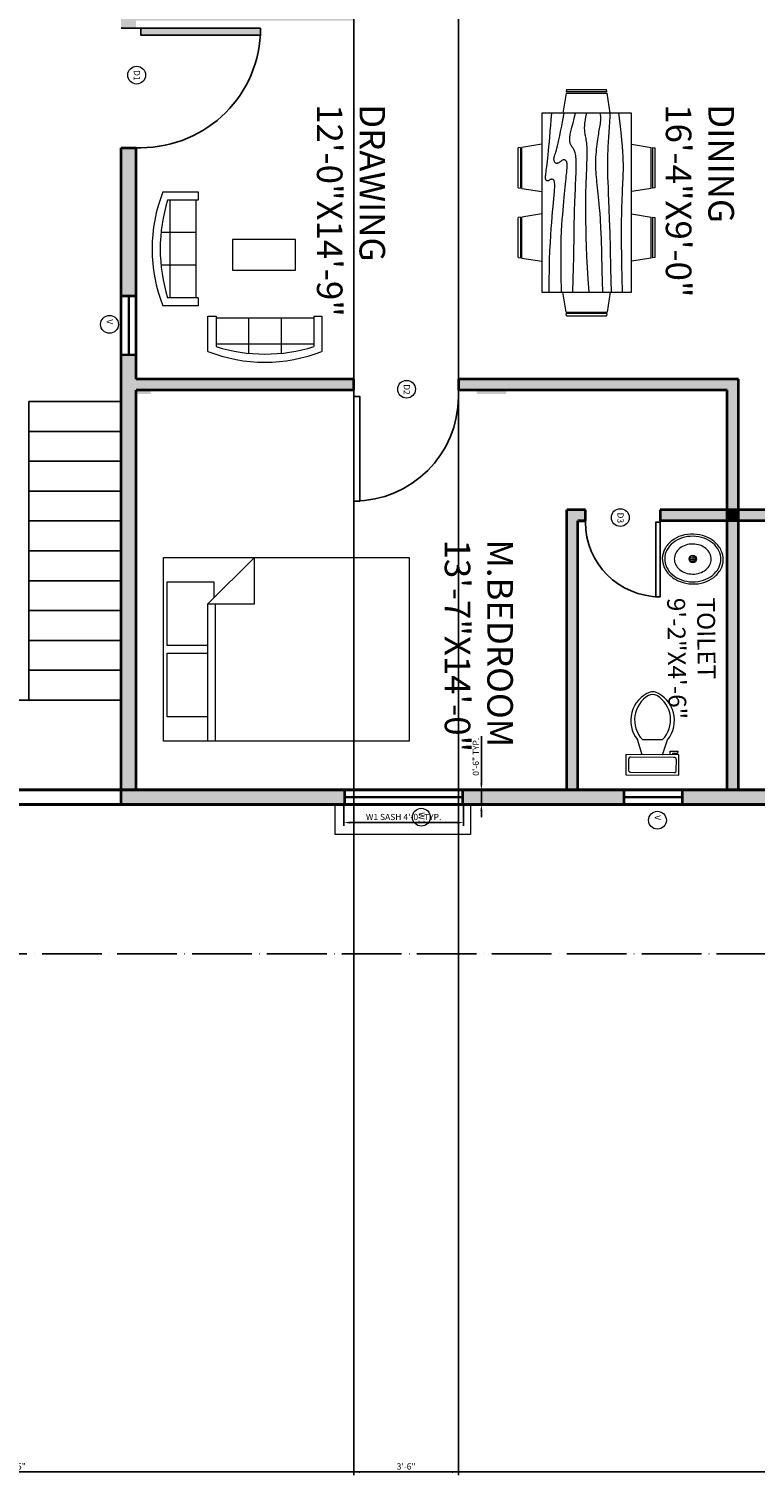
# Model space of a CAD drawing. Units: inches. Extents: x 7028582 to 7030319, y 63109697 to 63111305.
# Tile 6 of 18: x 7029711 to 7030003, y 63109697 to 63110278. Entities that reach past the tile are written whole.
import ezdxf

# ---------------------------------------------------------------- set-up
doc = ezdxf.new("R2010")
doc.units = ezdxf.units.IN
doc.linetypes.add('ACAD_ISO04W100', pattern=[30, 24, -3, 0, -3])
for name, color, linetype, lineweight in [('A-AREA-IDEN', 7, 'Continuous', 18), ('A-DOOR-IDEN', 20, 'Continuous', 13), ('A-FLOR-FIXT', 9, 'Continuous', 18), ('A-FLOR-STRS', 1, 'Continuous', 25), ('A-GLAZ-IDEN', 20, 'Continuous', 13), ('A-WALL-PATT', 8, 'Continuous', 13), ('C-ANNO-DIMS', 7, 'Continuous', 18), ('C-PROP', 1, 'ACAD_ISO04W100', 25), ('doors', 20, 'Continuous', 25), ('furniture', 9, 'Continuous', 18), ('S-COLS-PATT', 220, 'Continuous', 100), ('walls', 6, 'Continuous', 35), ('WINDOW SHADOW', 9, 'Continuous', 13), ('windows', 5, 'Continuous', 18)]:
    doc.layers.add(name, color=color, linetype=linetype, lineweight=lineweight)
doc.styles.get("Standard").update_dxf_attribs({"font": 'arial.ttf'})
doc.dimstyles.new('ISO-25', dxfattribs={"dimtxt": 2.5, "dimasz": 2.5, "dimexe": 1.25, "dimexo": 0.625, "dimtad": 1, "dimlunit": 4, "dimtxsty": 'Standard', "dimcen": 2.5, "dimadec": 0, "dimazin": 0, "dimtfac": 1, "dimtmove": 0, "dimatfit": 3, "dimfxl": 1, "dimarcsym": 0})

# ---------------------------------------------------------------- blocks, each defined once
blk = doc.blocks.new('*U2')
for p, q in [((0, 0), (0, -5)), ((30, 0), (30, -5))]:
    blk.add_line(p, q)
blk.add_lwpolyline([(0, 0), (0, 30), (1.75, 30), (1.75, 0)], close=True)
blk.add_arc((0, 0), 30, 0, 90)
blk = doc.blocks.new('Dining Set - 36 x 72 in.')
for p, q in [((-22.2343, 26.00059), (-23.4847, 17.99762)), ((-22.2304, 26), (-5.7608, 26)), ((-22, 27.5), (-22.1562, 26.50042)), ((-5.8416, 26.5), (-22.1534, 26.5)), ((-22, 27.5), (-6, 27.5)), ((-5.8437, 26.49966), (-6, 27.5)), ((-4.5152, 17.99762), (-5.7655, 25.99926)), ((5.7657, 26.00059), (4.5153, 17.99762)), ((5.7696, 26), (22.2392, 26)), ((6, 27.5), (5.8438, 26.50042)), ((22.1584, 26.5), (5.8466, 26.5)), ((6, 27.5), (22, 27.5)), ((22.1563, 26.49966), (22, 27.5)), ((23.4848, 17.99762), (22.2345, 25.99926)), ((36, 18), (-36, 18)), ((-36, 18), (-36, -18)), ((36, -18), (36, 18)), ((-45.5, 8), (-44.5004, 8.15617)), ((-45.5, 8), (-45.5, -8)), ((-44.5, -8.15843), (-44.5, 8.15338)), ((-44.0006, 8.23428), (-35.9976, 9.48474)), ((-44, 8.23041), (-44, -8.23915)), ((44.0006, 8.23428), (35.9976, 9.48474)), ((44, 8.23041), (44, -8.23915)), ((44.5, -8.15843), (44.5, 8.15338)), ((45.5, 8), (44.5005, 8.15617)), ((45.5, 8), (45.5, -8)), ((-44.4997, -8.15631), (-45.5, -8)), ((-35.9976, -9.48476), (-43.9993, -8.2345)), ((35.9976, -9.48476), (43.9993, -8.2345)), ((44.4997, -8.15631), (45.5, -8)), ((-36, -18), (36, -18)), ((-22.2343, -26.0006), (-23.4847, -17.99762)), ((-4.5152, -17.99762), (-5.7655, -25.99928)), ((5.7657, -26.0006), (4.5153, -17.99762)), ((23.4848, -17.99762), (22.2345, -25.99928)), ((-22.2304, -26), (-5.7608, -26)), ((-22, -27.5), (-22.1562, -26.50044)), ((-5.8416, -26.5), (-22.1534, -26.5)), ((-22, -27.5), (-6, -27.5)), ((-5.8437, -26.49967), (-6, -27.5)), ((5.7696, -26), (22.2392, -26)), ((6, -27.5), (5.8438, -26.50044)), ((22.1584, -26.5), (5.8466, -26.5)), ((6, -27.5), (22, -27.5)), ((22.1563, -26.49967), (22, -27.5))]:
    blk.add_line(p, q)
for points in [[(-36, 15), (-31.1772, 14.97754), (-26.8079, 14.91406), (-22.8538, 14.81543), (-19.276, 14.6875), (-16.0362, 14.53613), (-13.0957, 14.36718), (-10.4159, 14.18652), (-7.9583, 14), (-5.6904, 13.81315), (-3.6035, 13.63021), (-1.6954, 13.45508), (0.0365, 13.29166), (1.5945, 13.14388), (2.9811, 13.01562), (4.1988, 12.9108), (5.25, 12.83333), (6.1393, 12.78613), (6.8802, 12.76823), (7.4883, 12.77767), (7.9792, 12.8125), (8.3685, 12.87077), (8.6719, 12.95052), (8.9049, 13.0498), (9.0833, 13.16666), (9.2205, 13.29899), (9.3216, 13.44401), (9.3895, 13.59879), (9.4271, 13.76041), (9.4373, 13.92594), (9.4232, 14.09245), (9.3875, 14.257), (9.3333, 14.41666), (9.2638, 14.56917), (9.1836, 14.71484), (9.0975, 14.85465), (9.0104, 14.98958), (8.9272, 15.1206), (8.8529, 15.2487), (8.7922, 15.37483), (8.75, 15.5), (8.7305, 15.62467), (8.7344, 15.74739), (8.7617, 15.86621), (8.8125, 15.97916), (8.8867, 16.08431), (8.9844, 16.17968), (9.1055, 16.26334), (9.25, 16.33333), (9.4189, 16.38802), (9.6172, 16.42708), (9.8506, 16.45052), (10.125, 16.45833), (10.4463, 16.45052), (10.8203, 16.42708), (11.2529, 16.38802), (11.75, 16.33333), (12.3184, 16.26318), (12.9694, 16.17838), (13.7151, 16.07991), (14.5677, 15.96875), (15.5395, 15.84586), (16.6426, 15.71224), (17.8893, 15.56884), (19.2917, 15.41666), (20.859, 15.25667), (22.5879, 15.08984), (24.4721, 14.91715), (26.5052, 14.73958), (28.6809, 14.5581), (30.9929, 14.3737), (33.4347, 14.18733), (36, 14)], [(-36, 10), (-28.9766, 10.14274), (-23.1725, 10.20442), (-18.4241, 10.19775), (-14.5677, 10.13541), (-11.4399, 10.03011), (-8.877, 9.89453), (-6.7154, 9.74137), (-4.7917, 9.58333), (-2.9698, 9.43082), (-1.2246, 9.28515), (0.4415, 9.14534), (2.026, 9.01041), (3.5266, 8.87939), (4.9408, 8.7513), (6.266, 8.62516), (7.5, 8.5), (8.6411, 8.37549), (9.6914, 8.2539), (10.6538, 8.13818), (11.5312, 8.03125), (12.3267, 7.93603), (13.043, 7.85547), (13.6831, 7.79248), (14.25, 7.75), (14.7471, 7.7303), (15.1797, 7.73307), (15.5537, 7.75732), (15.875, 7.80208), (16.1494, 7.86637), (16.3828, 7.94922), (16.5811, 8.04964), (16.75, 8.16666), (16.8944, 8.29915), (17.0143, 8.44531), (17.1089, 8.60319), (17.1771, 8.77083), (17.218, 8.94629), (17.2305, 9.1276), (17.2137, 9.31282), (17.1667, 9.5), (17.0895, 9.6875), (16.987, 9.875), (16.8649, 10.0625), (16.7292, 10.25), (16.5856, 10.4375), (16.4401, 10.625), (16.2985, 10.8125), (16.1667, 11), (16.05, 11.18733), (15.9518, 11.3737), (15.8752, 11.5581), (15.8229, 11.73958), (15.798, 11.91715), (15.8034, 12.08984), (15.842, 12.25667), (15.9167, 12.41666), (16.0295, 12.56836), (16.1784, 12.70833), (16.3605, 12.83268), (16.5729, 12.9375), (16.8127, 13.01888), (17.0768, 13.07291), (17.3625, 13.0957), (17.6667, 13.08333), (17.9894, 13.03312), (18.3418, 12.94726), (18.7382, 12.82918), (19.1927, 12.68229), (19.7195, 12.51001), (20.3327, 12.31575), (21.0465, 12.10294), (21.875, 11.875), (22.8357, 11.63354), (23.959, 11.37304), (25.2786, 11.08618), (26.8282, 10.76562), (28.6414, 10.40405), (30.752, 9.99414), (33.1936, 9.52856), (36, 9)], [(-36, 5.5), (-30.7157, 5.3348), (-26.069, 5.20963), (-21.9946, 5.11767), (-18.4271, 5.05208), (-15.3009, 5.00602), (-12.5508, 4.97265), (-10.1112, 4.94515), (-7.9167, 4.91666), (-5.909, 4.88167), (-4.0586, 4.83984), (-2.3429, 4.79215), (-0.7396, 4.73958), (0.7739, 4.6831), (2.22, 4.6237), (3.6213, 4.56233), (5, 4.5), (6.373, 4.43782), (7.7344, 4.3776), (9.0723, 4.32129), (10.375, 4.27083), (11.6309, 4.22819), (12.8281, 4.19531), (13.9551, 4.17415), (15, 4.16666), (15.954, 4.17448), (16.819, 4.19791), (17.6001, 4.23698), (18.3021, 4.29166), (18.9299, 4.36198), (19.4883, 4.44791), (19.9823, 4.54948), (20.4167, 4.66666), (20.7969, 4.79899), (21.1302, 4.94401), (21.4245, 5.09879), (21.6875, 5.26041), (21.9271, 5.42594), (22.1511, 5.59245), (22.3672, 5.757), (22.5834, 5.91666), (22.8065, 6.06868), (23.0404, 6.21093), (23.2879, 6.34147), (23.5521, 6.45833), (23.8358, 6.55957), (24.142, 6.64323), (24.4735, 6.70735), (24.8334, 6.75), (25.2235, 6.76969), (25.642, 6.76692), (26.0858, 6.74267), (26.5521, 6.69791), (27.0379, 6.63362), (27.5404, 6.55078), (28.0565, 6.45036), (28.5834, 6.33333), (29.1242, 6.19987), (29.7071, 6.04687), (30.3661, 5.87044), (31.1354, 5.66666), (32.0493, 5.43164), (33.142, 5.16146), (34.4475, 4.85221), (36, 4.5)], [(-36, -1), (-30.7915, -0.6591), (-26.0195, -0.38216), (-21.6519, -0.16284), (-17.6563, 0.00521), (-14.0005, 0.12833), (-10.6523, 0.21289), (-7.5796, 0.26522), (-4.75, 0.29166), (-2.134, 0.29793), (0.2878, 0.28711), (2.5317, 0.26163), (4.6146, 0.22396), (6.5529, 0.17651), (8.3633, 0.12174), (10.0623, 0.06209), (11.6667, 0), (13.1899, -0.06201), (14.6341, -0.1211), (15.9982, -0.17432), (17.2813, -0.21875), (18.4823, -0.25147), (19.6003, -0.26953), (20.6343, -0.27002), (21.5834, -0.25), (22.4481, -0.20768), (23.2357, -0.14584), (23.9549, -0.06836), (24.6146, 0.02083), (25.2235, 0.11784), (25.7904, 0.21875), (26.3241, 0.31966), (26.8334, 0.41666), (27.3265, 0.50618), (27.8099, 0.58593), (28.2894, 0.65397), (28.7709, 0.70833), (29.2601, 0.74707), (29.763, 0.76823), (30.2855, 0.76985), (30.8334, 0.75), (31.4088, 0.70784), (31.9994, 0.64713), (32.589, 0.57275), (33.1615, 0.48958), (33.7008, 0.4025), (34.1908, 0.3164), (34.6153, 0.23616), (34.9584, 0.16666), (35.2099, 0.11165), (35.3848, 0.07031), (35.504, 0.04069), (35.5886, 0.02083), (35.6594, 0.00879), (35.7377, 0.0026), (35.8442, 0.00032), (36, 0)], [(-36, -6.5), (-27.1843, -6.31267), (-20.084, -6.1263), (-14.469, -5.9419), (-10.1094, -5.76042), (-6.7752, -5.58285), (-4.2363, -5.41016), (-2.2629, -5.24333), (-0.625, -5.08334), (0.8708, -4.93099), (2.2715, -4.78646), (3.5872, -4.64974), (4.8281, -4.52084), (6.0046, -4.39974), (7.127, -4.28646), (8.2053, -4.18099), (9.25, -4.08334), (10.2705, -3.99382), (11.2734, -3.91407), (12.2647, -3.84603), (13.25, -3.79167), (14.2354, -3.75293), (15.2266, -3.73177), (16.2295, -3.73015), (17.25, -3.75), (18.2912, -3.79248), (19.3451, -3.85547), (20.4009, -3.93604), (21.4479, -4.03125), (22.4754, -4.13819), (23.4727, -4.25391), (24.4289, -4.37549), (25.3334, -4.5), (26.1785, -4.62492), (26.9694, -4.74935), (27.7145, -4.87281), (28.4219, -4.99479), (29.1, -5.11483), (29.7572, -5.23242), (30.4016, -5.34709), (31.0417, -5.45834), (31.6837, -5.56437), (32.3262, -5.65821), (32.9658, -5.73153), (33.599, -5.77604), (34.2224, -5.78345), (34.8327, -5.74545), (35.4264, -5.65373), (36, -5.5)], [(-36, -10), (-26.4022, -9.81299), (-18.4675, -9.62891), (-11.9839, -9.45069), (-6.7396, -9.28125), (-2.5226, -9.12354), (0.8789, -8.98047), (3.6769, -8.85498), (6.0833, -8.75), (8.2767, -8.66765), (10.3021, -8.60677), (12.1712, -8.56543), (13.8958, -8.54167), (15.4876, -8.53353), (16.9583, -8.53907), (18.3197, -8.55632), (19.5834, -8.58334), (20.7616, -8.61841), (21.8685, -8.66081), (22.9188, -8.71004), (23.9271, -8.76563), (24.9081, -8.82707), (25.8763, -8.89388), (26.8465, -8.96558), (27.8334, -9.04167), (28.8474, -9.12118), (29.8828, -9.20117), (30.93, -9.27824), (31.9792, -9.34896), (33.0205, -9.40991), (34.0443, -9.45768), (35.0407, -9.48885), (36, -9.5)], [(-36, -14.5), (-30.0881, -14.33513), (-25.0332, -14.21224), (-20.7312, -14.12647), (-17.0781, -14.07292), (-13.97, -14.04671), (-11.3027, -14.04297), (-8.9724, -14.05681), (-6.875, -14.08334), (-4.9224, -14.11833), (-3.0905, -14.16016), (-1.3709, -14.20785), (0.2448, -14.26042), (1.7647, -14.3169), (3.1973, -14.3763), (4.5507, -14.43767), (5.8333, -14.5), (7.0554, -14.5621), (8.235, -14.62175), (9.3922, -14.67652), (10.5469, -14.72396), (11.7192, -14.76164), (12.929, -14.78711), (14.1965, -14.79794), (15.5417, -14.79167), (16.9933, -14.76424), (18.6152, -14.70508), (20.4804, -14.60197), (22.6615, -14.44271), (25.2312, -14.21509), (28.2624, -13.9069), (31.8277, -13.50594), (36, -13)]]:
    blk.add_lwpolyline(points)
blk = doc.blocks.new('Sofa - Roundback 7 ft.')
for p, q in [((-12.00002, -32.4421), (-12.00003, -6.5971)), ((11.99997, -32.4421), (11.99998, -6.5971)), ((-36.000027, -34), (-36.000027, -11.4696)), ((-35.999844, -13.3819), (35.9998, -13.3819)), ((35.99998, -34), (35.99998, -11.4696)), ((-36.000027, -32.4421), (35.99998, -32.4421))]:
    blk.add_line(p, q)
for points in [[(-36.000027, -34), (-42.000027, -34), (-42.000027, -8)], [(41.99998, -8), (41.99998, -34), (35.99998, -34)]]:
    blk.add_lwpolyline(points)
for centre, radius, start, end in [((0, -114.25), 114.25, 68.43141, 111.5686), ((-0.00001, -127.1968), 121.1968, 72.72033, 107.2797)]:
    blk.add_arc(centre, radius, start, end)
blk = doc.blocks.new('Toilet - top')
for p, q in [((9.5, -6), (9.5, -2)), ((-10, -8.5), (-8, -8.5)), ((-10, -9.5), (-10, -8.5)), ((-7, -9.5), (-10, -9.5)), ((-8, -8.5), (-8, -8)), ((-7, -8), (-7, -9.5)), ((-4, -8), (-6, -14)), ((4, -8), (6, -14)), ((4, -14), (-4, -14))]:
    blk.add_line(p, q)
blk.add_lwpolyline([(10.5, -8), (10.5, 0), (-10.5, 0), (-10.5, -8)], close=True)
for points in [[(-9.5, -2), (-9.5, -6)], [(8.5, -1), (-8.5, -1)], [(-8.5, -7), (8.5, -7)]]:
    blk.add_lwpolyline(points)
for centre, radius, start, end in [((-8.62, -1.88), 0.884, 81.8699, 188.1301), ((8.62, -1.88), 0.884, 351.8699, 98.1301), ((-8.62, -6.12), 0.884, 171.8699, 278.1301), ((8.62, -6.12), 0.884, 261.8699, 8.1301), ((3.52, -21.58), 12.17, 141.46911, 247.97143), ((4.2, -21.82), 11.33, 136.36773, 238.94682), ((-3.52, -21.58), 12.17, 292.02843, 38.53071), ((-4.2, -21.82), 11.33, 301.05301, 43.63209), ((0, -27.88), 4, 245.73182, 294.26817), ((0, -29), 4, 254.86053, 285.13947)]:
    blk.add_arc(centre, radius, start, end)
blk = doc.blocks.new('Sink - Oval top')
for p, q in [((-1, 0), (1, 0)), ((0, 1), (0, -1))]:
    blk.add_line(p, q)
for points in [[(-12.23, 0.39, 0.117634), (-11.46, -3.36, 0.104469), (-8.88, -6.8, 0.090016), (-5.08, -9.07, 0.08192), (-0.32, -10.02, 0.08192), (4.49, -9.38, 0.090016), (8.42, -7.36, 0.104469), (11.22, -4.09, 0.117634), (12.23, -0.39, 0.117634), (11.46, 3.36, 0.104469), (8.88, 6.8, 0.090016), (5.08, 9.07, 0.08192), (0.32, 10.02, 0.08192), (-4.49, 9.38, 0.090016), (-8.42, 7.36, 0.104469), (-11.22, 4.09, 0.117634)], [(-11.29, 0.16, 0.118622), (-10.52, -3.25, 0.104678), (-8.07, -6.36, 0.089562), (-4.54, -8.37, 0.081185), (-0.13, -9.15, 0.081185), (4.3, -8.49, 0.089562), (7.89, -6.58, 0.104678), (10.42, -3.55, 0.118622), (11.29, -0.16, 0.118622), (10.52, 3.25, 0.104678), (8.07, 6.36, 0.089562), (4.54, 8.37, 0.081185), (0.13, 9.15, 0.081185), (-4.3, 8.49, 0.089562), (-7.89, 6.58, 0.104678), (-10.42, 3.55, 0.118622)], [(-7.42, 0.08, 0.118283), (-6.91, -2.17, 0.104607), (-5.29, -4.21, 0.089718), (-2.97, -5.53, 0.081436), (-0.07, -6.04, 0.081436), (2.84, -5.59, 0.089718), (5.2, -4.33, 0.104607), (6.86, -2.32, 0.118283), (7.42, -0.08, 0.118283), (6.91, 2.17, 0.104607), (5.29, 4.21, 0.089718), (2.97, 5.53, 0.081436), (0.07, 6.04, 0.081436), (-2.84, 5.59, 0.089718), (-5.2, 4.33, 0.104607), (-6.86, 2.32, 0.118283)]]:
    blk.add_lwpolyline(points, format="xyb", close=True)
for radius in [1.5, 1]:
    blk.add_circle((0, 0), radius)
blk = doc.blocks.new('Bed - Queen')
for p, q in [((0, -80.00003), (0, 0)), ((0, 0), (59.99999, 0)), ((59.99999, 0), (59.99999, -80.00003)), ((7.99999, -1.2), (28.79998, -1.2)), ((7.99999, -14.4), (7.99999, -1.2)), ((28.79998, -1.2), (28.79998, -14.4)), ((31.19999, -1.2), (51.99999, -1.2)), ((31.19999, -14.4), (31.19999, -1.2)), ((51.99999, -1.2), (51.99999, -16.4)), ((0, -14.4), (44.8, -14.4)), ((44.8, -16.8), (0, -16.8)), ((59.99999, -29.6), (44.8, -14.4)), ((44.8, -14.4), (44.8, -29.6)), ((51.99999, -16.4), (46.79936, -16.4)), ((44.8, -29.6), (59.99999, -29.6)), ((59.99999, -80.00003), (0, -80.00003))]:
    blk.add_line(p, q)
blk = doc.blocks.new('WIN-SASH-24')
for p, q in [((24.05, 6), (0, 6)), ((0.5, 6), (0.5, 0)), ((23.55, 0), (23.55, 6)), ((0, 0), (24.05, 0)), ((23.55, 3.2), (0.5, 3.2)), ((23.55, 2.8), (0.5, 2.8))]:
    blk.add_line(p, q)
blk = doc.blocks.new('WIN-SASH-48')
for p, q in [((48.05, 6), (0, 6)), ((0.5, 6), (0.5, 0)), ((47.55, 0), (47.55, 6)), ((47.55, 3.2), (0.5, 3.2)), ((47.55, 2.8), (0.5, 2.8)), ((0, 0), (48.05, 0))]:
    blk.add_line(p, q)
blk = doc.blocks.new('WINDOW-SHADE-HEAD-54')
for p, q in [((0, 0), (0, 12)), ((54.39, 12), (54.39, 0)), ((54.39, 0), (0, 0))]:
    blk.add_line(p, q)
blk = doc.blocks.new('TABLE-COFFEE-RECT')
blk.add_lwpolyline([(25.34, 12.34), (0, 12.34), (0, 0), (25.34, 0)], close=True)
blk = doc.blocks.new('TAG-D1-MT-R')
blk.add_circle((3.58, 3.58), 3.58)
at = {"insert": (4.93, 5.6), "char_height": 2.5, "attachment_point": 1, "rotation": 270}
blk.add_mtext_dynamic_manual_height_columns('D1', width=2.5021, gutter_width=12.5, heights=[0], dxfattribs=at)
blk = doc.blocks.new('TAG-D2-MT-R')
blk.add_circle((3.58, 3.58), 3.58)
at = {"insert": (4.93, 5.6), "char_height": 2.5, "attachment_point": 1, "rotation": 270}
blk.add_mtext_dynamic_manual_height_columns('D2', width=2.5021, gutter_width=12.5, heights=[0], dxfattribs=at)
blk = doc.blocks.new('TAG-D3-MT-R')
blk.add_circle((3.58, 3.58), 3.58)
at = {"insert": (4.93, 5.6), "char_height": 2.5, "attachment_point": 1, "rotation": 270}
blk.add_mtext_dynamic_manual_height_columns('D3', width=2.5021, gutter_width=12.5, heights=[0], dxfattribs=at)
blk = doc.blocks.new('TAG-V-MT-R')
blk.add_circle((3.58, 3.58), 3.58)
at = {"insert": (4.93, 5.6), "char_height": 2.5, "attachment_point": 1, "rotation": 270}
blk.add_mtext_dynamic_manual_height_columns('V', width=2.5021, gutter_width=12.5, heights=[0], dxfattribs=at)
blk = doc.blocks.new('TAG-W1-MT-R')
blk.add_circle((3.58, 3.58), 3.58)
at = {"insert": (4.93, 5.6), "char_height": 2.5, "attachment_point": 1, "rotation": 270}
blk.add_mtext_dynamic_manual_height_columns('W1', width=2.5021, gutter_width=12.5, heights=[0], dxfattribs=at)
blk = doc.blocks.new('*D67')
at = {"layer": 'C-ANNO-DIMS', "color": 0, "lineweight": -2, "transparency": 16777216}
for p, q in [((7029837.68, 63109965.93), (7029837.68, 63109958.1)), ((7029885.73, 63109965.93), (7029885.73, 63109958.1)), ((7029840.18, 63109959.35), (7029883.23, 63109959.35))]:
    blk.add_line(p, q, dxfattribs=at)
at = {"layer": 'C-ANNO-DIMS', "color": 0, "lineweight": 100, "transparency": 16777216}
for points in [[(7029840.18, 63109959.77), (7029840.18, 63109958.93), (7029837.68, 63109959.35)], [(7029883.23, 63109959.77), (7029883.23, 63109958.93), (7029885.73, 63109959.35)]]:
    blk.add_solid(points, dxfattribs=at)
at = {"layer": 'Defpoints', "color": 0, "lineweight": 100, "transparency": 16777216}
for p in [(7029837.68, 63109966.56), (7029885.73, 63109966.56), (7029885.73, 63109959.35)]:
    blk.add_point(p, dxfattribs=at)
at = {"layer": 'C-ANNO-DIMS', "color": 0, "transparency": 16777216, "insert": (7029861.7, 63109961.27), "char_height": 2.5, "attachment_point": 5}
blk.add_mtext('W1 SASH 4\'-0" TYP.', dxfattribs=at)
blk = doc.blocks.new('*D68')
at = {"layer": 'C-ANNO-DIMS', "color": 0, "lineweight": -2, "transparency": 16777216}
for p, q in [((7029892.93, 63109975.06), (7029892.93, 63109994.05)), ((7029886.35, 63109972.56), (7029894.18, 63109972.56)), ((7029892.93, 63109966.56), (7029892.93, 63109972.56)), ((7029886.35, 63109966.56), (7029894.18, 63109966.56)), ((7029892.93, 63109964.06), (7029892.93, 63109961.56))]:
    blk.add_line(p, q, dxfattribs=at)
at = {"layer": 'C-ANNO-DIMS', "color": 0, "lineweight": 100, "transparency": 16777216}
for points in [[(7029892.52, 63109975.06), (7029893.35, 63109975.06), (7029892.93, 63109972.56)], [(7029892.52, 63109964.06), (7029893.35, 63109964.06), (7029892.93, 63109966.56)]]:
    blk.add_solid(points, dxfattribs=at)
at = {"layer": 'Defpoints', "color": 0, "lineweight": 100, "transparency": 16777216}
for p in [(7029885.73, 63109972.56), (7029892.93, 63109972.56), (7029885.73, 63109966.56)]:
    blk.add_point(p, dxfattribs=at)
at = {"layer": 'C-ANNO-DIMS', "color": 0, "transparency": 16777216, "insert": (7029891.03, 63109985.8), "char_height": 2.5, "attachment_point": 5, "rotation": 90}
blk.add_mtext('0\'-6" TYP.', dxfattribs=at)
blk = doc.blocks.new('*D99')
at = {"layer": 'C-ANNO-DIMS', "color": 0, "lineweight": -2, "transparency": 16777216}
for p, q in [((7029234.71, 63109965.93), (7029234.71, 63109697.14)), ((7030175.71, 63109965.93), (7030175.71, 63109697.14)), ((7029237.21, 63109698.39), (7030173.21, 63109698.39))]:
    blk.add_line(p, q, dxfattribs=at)
at = {"layer": 'C-ANNO-DIMS', "color": 0, "lineweight": 100, "transparency": 16777216}
for points in [[(7029237.21, 63109698.8), (7029237.21, 63109697.97), (7029234.71, 63109698.39)], [(7030173.21, 63109698.8), (7030173.21, 63109697.97), (7030175.71, 63109698.39)]]:
    blk.add_solid(points, dxfattribs=at)
at = {"layer": 'Defpoints', "color": 0, "lineweight": 100, "transparency": 16777216}
for p in [(7029234.71, 63109966.56), (7030175.71, 63109966.56), (7030175.71, 63109698.39)]:
    blk.add_point(p, dxfattribs=at)
at = {"layer": 'C-ANNO-DIMS', "color": 0, "transparency": 16777216, "insert": (7029705.21, 63109700.29), "char_height": 2.5, "attachment_point": 5}
blk.add_mtext('78\'-5"', dxfattribs=at)
blk = doc.blocks.new('*D105')
at = {"layer": 'C-ANNO-DIMS', "color": 0, "lineweight": -2, "transparency": 16777216}
for p, q in [((7029841.68, 63110859.93), (7029841.68, 63109697.14)), ((7029883.68, 63110859.93), (7029883.68, 63109697.14)), ((7029844.18, 63109698.39), (7029881.18, 63109698.39))]:
    blk.add_line(p, q, dxfattribs=at)
at = {"layer": 'C-ANNO-DIMS', "color": 0, "lineweight": 100, "transparency": 16777216}
for points in [[(7029844.18, 63109698.8), (7029844.18, 63109697.97), (7029841.68, 63109698.39)], [(7029881.18, 63109698.8), (7029881.18, 63109697.97), (7029883.68, 63109698.39)]]:
    blk.add_solid(points, dxfattribs=at)
at = {"layer": 'Defpoints', "color": 0, "lineweight": 100, "transparency": 16777216}
for p in [(7029841.68, 63110860.56), (7029883.68, 63110860.56), (7029883.68, 63109698.39)]:
    blk.add_point(p, dxfattribs=at)
at = {"layer": 'C-ANNO-DIMS', "color": 0, "transparency": 16777216, "insert": (7029862.68, 63109700.29), "char_height": 2.5, "attachment_point": 5}
blk.add_mtext('3\'-6"', dxfattribs=at)
blk = doc.blocks.new('*D110')
at = {"layer": 'C-ANNO-DIMS', "color": 0, "lineweight": -2, "transparency": 16777216}
for p, q in [((7029747.58, 63110008.56), (7028586.23, 63110008.56)), ((7028587.48, 63110006.06), (7028587.48, 63109975.06)), ((7029747.58, 63109972.56), (7028586.23, 63109972.56))]:
    blk.add_line(p, q, dxfattribs=at)
at = {"layer": 'C-ANNO-DIMS', "color": 0, "lineweight": 100, "transparency": 16777216}
for points in [[(7028587.06, 63110006.06), (7028587.89, 63110006.06), (7028587.48, 63110008.56)], [(7028587.06, 63109975.06), (7028587.89, 63109975.06), (7028587.48, 63109972.56)]]:
    blk.add_solid(points, dxfattribs=at)
at = {"layer": 'Defpoints', "color": 0, "lineweight": 100, "transparency": 16777216}
for p in [(7029748.21, 63110008.56), (7028587.48, 63109972.56), (7029748.21, 63109972.56)]:
    blk.add_point(p, dxfattribs=at)
at = {"layer": 'C-ANNO-DIMS', "color": 0, "transparency": 16777216, "insert": (7028585.57, 63109990.56), "char_height": 2.5, "attachment_point": 5, "rotation": 90}
blk.add_mtext('3\'-0"', dxfattribs=at)

msp = doc.modelspace()

# ---------------------------------------------------------------- hatches: boundary and pattern name
at = {"layer": 'A-WALL-PATT'}
h = msp.add_hatch(color=256, dxfattribs=at)
h.dxf.hatch_style = 1
h.paths.add_polyline_path([(7029754.205, 63110278.557), (7029756.205, 63110278.557), (7029804.205, 63110278.557), (7029804.205, 63110275.757), (7029756.205, 63110275.757), (7029756.205, 63110278.557), (7029748.205, 63110278.557), (7029748.205, 63110448.057), (7029754.205, 63110448.057), (7029754.205, 63110286.057), (7029841.685, 63110286.057), (7029841.685, 63110288.557), (7029841.685, 63110330.557), (7029844.135, 63110330.557), (7029844.135, 63110288.557), (7029841.685, 63110288.557), (7029841.685, 63110281.557), (7029754.205, 63110281.557)])
h = msp.add_hatch(color=256, dxfattribs=at)
h.dxf.hatch_style = 1
h.paths.add_polyline_path([(7029754.205, 63110230.557), (7029748.205, 63110230.557), (7029748.205, 63110171.186), (7029754.205, 63110171.186)])
h = msp.add_hatch(color=256, dxfattribs=at)
h.dxf.hatch_style = 1
h.paths.add_polyline_path([(7029841.685, 63110137.557), (7029754.205, 63110137.557), (7029754.205, 63110147.137), (7029748.205, 63110147.137), (7029748.205, 63109966.557), (7029837.679, 63109966.557), (7029837.679, 63109972.557), (7029754.205, 63109972.557), (7029754.205, 63110133.057), (7029841.685, 63110133.057)])
h = msp.add_hatch(color=256, dxfattribs=at)
h.dxf.hatch_style = 1
h.paths.add_polyline_path([(7029996.205, 63110137.557), (7029883.685, 63110137.557), (7029883.685, 63110133.057), (7029991.705, 63110133.057), (7029991.705, 63110085.057), (7029996.205, 63110085.057)])
h = msp.add_hatch(color=256, dxfattribs=at)
h.dxf.hatch_style = 1
h.paths.add_polyline_path([(7029949.931, 63109972.557), (7029931.705, 63109972.557), (7029931.705, 63110080.557), (7029934.705, 63110080.557), (7029934.705, 63110085.057), (7029927.205, 63110085.057), (7029927.205, 63109972.557), (7029885.727, 63109972.557), (7029885.727, 63109966.557), (7029949.931, 63109966.557)])
h = msp.add_hatch(color=256, dxfattribs=at)
h.dxf.hatch_style = 1
h.paths.add_polyline_path([(7029991.705, 63110085.057), (7029964.705, 63110085.057), (7029964.705, 63110080.557), (7029991.705, 63110080.557)])
h = msp.add_hatch(color=256, dxfattribs=at)
h.dxf.hatch_style = 1
h.paths.add_polyline_path([(7029996.205, 63110085.057), (7029991.705, 63110085.057), (7029991.705, 63110080.557), (7029996.205, 63110080.557)])
h = msp.add_hatch(color=256, dxfattribs=at)
h.dxf.hatch_style = 1
h.paths.add_polyline_path([(7030049.705, 63110085.057), (7029996.205, 63110085.057), (7029996.205, 63110080.557), (7030045.205, 63110080.557), (7030045.205, 63110077.557), (7030049.705, 63110077.557)])
h = msp.add_hatch(color=256, dxfattribs=at)
h.dxf.hatch_style = 1
h.paths.add_polyline_path([(7029996.205, 63110080.557), (7029991.705, 63110080.557), (7029991.705, 63109972.557), (7029973.979, 63109972.557), (7029973.979, 63109966.557), (7030008.697, 63109966.557), (7030008.697, 63109972.557), (7029996.205, 63109972.557)])
at = {"layer": 'S-COLS-PATT'}
h = msp.add_hatch(color=256, dxfattribs=at)
h.dxf.hatch_style = 1
h.paths.add_polyline_path([(7029760.108, 63110137.557), (7029748.205, 63110137.557), (7029748.205, 63110131.557), (7029760.108, 63110131.557)])
h = msp.add_hatch(color=256, dxfattribs=at)
h.dxf.hatch_style = 1
h.paths.add_polyline_path([(7029902.915, 63110137.557), (7029891, 63110137.557), (7029891, 63110131.557), (7029902.915, 63110131.557)])
h = msp.add_hatch(color=256, dxfattribs=at)
h.dxf.hatch_style = 1
h.paths.add_polyline_path([(7029760.108, 63109972.505), (7029748.205, 63109972.505), (7029748.205, 63109966.505), (7029760.108, 63109966.505)])
h = msp.add_hatch(color=256, dxfattribs=at)
h.dxf.hatch_style = 1
h.paths.add_polyline_path([(7029902.915, 63109972.505), (7029891, 63109972.505), (7029891, 63109966.505), (7029902.915, 63109966.505)])

# ---------------------------------------------------------------- linework, layer by layer
at = {"layer": 'A-FLOR-STRS'}
for p, q in [((7029748.205, 63110128.557), (7029711.205, 63110128.557)), ((7029711.205, 63110008.557), (7029711.205, 63110128.557)), ((7029748.205, 63110116.557), (7029711.205, 63110116.557)), ((7029748.205, 63110104.557), (7029711.205, 63110104.557)), ((7029748.205, 63110092.557), (7029711.205, 63110092.557)), ((7029748.205, 63110080.557), (7029711.205, 63110080.557)), ((7029748.205, 63110068.557), (7029711.205, 63110068.557)), ((7029748.205, 63110056.557), (7029711.205, 63110056.557)), ((7029748.205, 63110044.557), (7029711.205, 63110044.557)), ((7029748.205, 63110032.557), (7029711.205, 63110032.557)), ((7029748.205, 63110020.557), (7029711.205, 63110020.557)), ((7029748.205, 63110008.557), (7029662.205, 63110008.557))]:
    msp.add_line(p, q, dxfattribs=at)
at = {"layer": 'C-PROP'}
msp.add_line((7029174.705, 63109906.557), (7030235.705, 63109906.557), dxfattribs=at)
at = {"layer": 'walls'}
for p, q in [((7029748.205, 63109966.557), (7029748.205, 63110230.557)), ((7029748.205, 63110230.557), (7029754.205, 63110230.557)), ((7029754.205, 63110137.557), (7029754.205, 63110230.557)), ((7029841.685, 63110137.557), (7029754.205, 63110137.557)), ((7029841.685, 63110133.057), (7029841.685, 63110137.557)), ((7029883.685, 63110137.557), (7029883.685, 63110133.057)), ((7029996.205, 63110137.557), (7029883.685, 63110137.557)), ((7029996.205, 63109972.557), (7029996.205, 63110137.557)), ((7029754.205, 63109972.557), (7029754.205, 63110133.057)), ((7029841.685, 63110133.057), (7029754.205, 63110133.057)), ((7029991.705, 63110133.057), (7029883.685, 63110133.057)), ((7029991.705, 63109972.557), (7029991.705, 63110133.057)), ((7029927.205, 63109972.557), (7029927.205, 63110085.057)), ((7029934.705, 63110085.057), (7029927.205, 63110085.057)), ((7029934.705, 63110080.557), (7029934.705, 63110085.057)), ((7030049.705, 63110085.057), (7029964.705, 63110085.057)), ((7029964.705, 63110085.057), (7029964.705, 63110080.557)), ((7029931.705, 63109972.557), (7029931.705, 63110080.557)), ((7029934.705, 63110080.557), (7029931.705, 63110080.557)), ((7029931.705, 63110080.557), (7029934.705, 63110080.557)), ((7030045.205, 63110080.557), (7029964.705, 63110080.557)), ((7029240.705, 63109972.557), (7030169.705, 63109972.557)), ((7030169.705, 63109972.557), (7029240.705, 63109972.557)), ((7029748.205, 63109972.557), (7029662.205, 63109972.557)), ((7029748.205, 63109972.557), (7029662.205, 63109972.557)), ((7029927.205, 63109972.557), (7029754.205, 63109972.557)), ((7029991.705, 63109972.557), (7029931.705, 63109972.557)), ((7030045.205, 63109972.557), (7029996.205, 63109972.557)), ((7029234.705, 63109966.557), (7030175.705, 63109966.557)), ((7030175.705, 63109966.557), (7029234.705, 63109966.557)), ((7030175.705, 63109966.557), (7029748.205, 63109966.557))]:
    msp.add_line(p, q, dxfattribs=at)
at = {"layer": 'windows'}
for p, q in [((7029754.205, 63110171.186), (7029748.205, 63110171.186)), ((7029748.205, 63110147.137), (7029754.205, 63110147.137)), ((7029837.679, 63109972.557), (7029837.679, 63109966.557)), ((7029885.727, 63109966.557), (7029885.727, 63109972.557)), ((7029949.931, 63109972.557), (7029949.931, 63109966.557)), ((7029973.979, 63109966.557), (7029973.979, 63109972.557))]:
    msp.add_line(p, q, dxfattribs=at)

# ---------------------------------------------------------------- block references
at = {"layer": 'A-DOOR-IDEN'}
for name, p in [('TAG-D1-MT-R', (7029750.898, 63110256.142)), ('TAG-D2-MT-R', (7029859.301, 63110129.893)), ('TAG-D3-MT-R', (7029945.138, 63110078.328))]:
    msp.add_blockref(name, p, dxfattribs=at)
at = {"layer": 'A-FLOR-FIXT'}
msp.add_blockref('Sink - Oval top', (7029977.829, 63110065.243), dxfattribs=at)
at = {"layer": 'A-FLOR-FIXT', "xscale": 1.013555723357934, "yscale": 1.013555723357934, "zscale": 1.013555723357934, "rotation": 179.7253796204469}
msp.add_blockref('Toilet - top', (7029961.58, 63109978.497), dxfattribs=at)
at = {"layer": 'A-GLAZ-IDEN'}
for name, p in [('TAG-V-MT-R', (7029739.972, 63110155.979)), ('TAG-W1-MT-R', (7029865.247, 63109957.914)), ('TAG-V-MT-R', (7029960.057, 63109956.713))]:
    msp.add_blockref(name, p, dxfattribs=at)
at = {"layer": 'doors'}
for p, xscale, yscale, zscale, rotation in [((7029756.205, 63110278.557), 1.599999999999999, 1.599999999999999, 1.599999999999999, 270), ((7029841.685, 63110130.557), -1.399999999999999, 1.399999999999999, 1.399999999999999, 180)]:
    msp.add_blockref('*U2', p, dxfattribs=dict(at, xscale=xscale, yscale=yscale, zscale=zscale, rotation=rotation))
at = {"layer": 'doors', "rotation": 180}
msp.add_blockref('*U2', (7029964.705, 63110080.057), dxfattribs=at)
at = {"layer": 'furniture', "rotation": 90}
msp.add_blockref('Dining Set - 36 x 72 in.', (7029935.163, 63110208.448), dxfattribs=at)
at = {"layer": 'furniture'}
for name, p, xscale, yscale, zscale, rotation in [('Sofa - Roundback 7 ft.', (7029760.658, 63110189.875), 0.5455524879488546, 0.5455524879488546, 0.5455524879488546, 90), ('Sofa - Roundback 7 ft.', (7029805.982, 63110144.346), 0.5455524879488546, 0.5455524879488546, 0.5455524879488546, 180), ('Bed - Queen', (7029765.303, 63109992.002), 1.232093012797833, 1.232093012797833, 1.232093012797833, 89.99999999999999)]:
    msp.add_blockref(name, p, dxfattribs=dict(at, xscale=xscale, yscale=yscale, zscale=zscale, rotation=rotation))
msp.add_blockref('TABLE-COFFEE-RECT', (7029792.974, 63110181.346), dxfattribs=at)
at = {"layer": 'WINDOW SHADOW'}
msp.add_blockref('WINDOW-SHADE-HEAD-54', (7029834.199, 63109954.557), dxfattribs=at)
at = {"layer": 'windows', "rotation": 89.99999995093432}
msp.add_blockref('WIN-SASH-24', (7029754.205, 63110147.137), dxfattribs=at)
at = {"layer": 'windows'}
for name, p in [('WIN-SASH-48', (7029837.679, 63109966.557)), ('WIN-SASH-24', (7029949.931, 63109966.557))]:
    msp.add_blockref(name, p, dxfattribs=at)

# ---------------------------------------------------------------- texts
at = {"layer": 'A-AREA-IDEN', "attachment_point": 1}
for s, width, gutter_width, insert, char_height, rotation in [('DRAWING\\P12\'-0"X14\'-9"', 82.04322, 51.315, (7029854.241, 63110248.03), 10.26307, 270), ('DINING\\P16\'-4"X9\'-0"', 82.04322, 51.315, (7029994.376, 63110248.03), 10.26307, 270), ('M.BEDROOM\\P13\'-7"X14\'-0"', 82.04322, 51.315, (7029905.577, 63110073.083), 10.26307, 270), ('TOILET\\P9\'-2"X4\'-6"', 42.97461, 35.821, (7029986.665, 63110049.835), 7.16426, 270.646399)]:
    msp.add_mtext_dynamic_manual_height_columns(s, width=width, gutter_width=gutter_width, heights=[0], dxfattribs=dict(at, insert=insert, char_height=char_height, rotation=rotation))

# ---------------------------------------------------------------- dimensions: what is measured, and where the dimension line sits
at = {"layer": 'C-ANNO-DIMS'}
for base, p1, p2, picture, middle in [((7029883.685, 63109698.385), (7029841.685, 63110860.557), (7029883.685, 63110860.557), '*D105', (7029862.685, 63109700.288)), ((7030175.705, 63109698.385), (7029234.705, 63109966.557), (7030175.705, 63109966.557), '*D99', (7029705.205, 63109700.287))]:
    dim = msp.add_linear_dim(base=base, p1=p1, p2=p2, dimstyle='ISO-25', override={"dimdec": 1, "dimlfac": 1, "dimrnd": 0, "dimzin": 1, "dimdsep": 46, "dimlunit": 4, "dimfrac": 2}, dxfattribs=at)
    dim.commit()
    dim.dimension.update_dxf_attribs({"geometry": picture, "text_midpoint": middle})
dim = msp.add_linear_dim(base=(7028587.475, 63109972.557), p1=(7029748.205, 63110008.557), p2=(7029748.205, 63109972.557), angle=90, dimstyle='ISO-25', override={"dimdec": 1, "dimlfac": 1, "dimrnd": 0, "dimzin": 1, "dimdsep": 46, "dimlunit": 4, "dimfrac": 2}, dxfattribs=at)
dim.commit()
dim.dimension.update_dxf_attribs({"geometry": '*D110', "text_midpoint": (7028585.573, 63109990.557)})
dim = msp.add_linear_dim(base=(7029892.934, 63109972.557), p1=(7029885.727, 63109966.557), p2=(7029885.727, 63109972.557), angle=90, text='<> TYP.', dimstyle='ISO-25', override={"dimdec": 1, "dimlfac": 1, "dimrnd": 0, "dimzin": 1, "dimdsep": 46, "dimlunit": 4, "dimfrac": 2}, dxfattribs=at)
dim.commit()
dim.dimension.update_dxf_attribs({"geometry": '*D68', "text_midpoint": (7029891.033, 63109985.801)})
dim = msp.add_linear_dim(base=(7029885.727, 63109959.349), p1=(7029837.679, 63109966.557), p2=(7029885.727, 63109966.557), text='W1 SASH <> TYP.', dimstyle='ISO-25', override={"dimdec": 1, "dimlfac": 1, "dimrnd": 0, "dimzin": 1, "dimdsep": 46, "dimlunit": 4, "dimfrac": 2}, dxfattribs=at)
dim.commit()
dim.dimension.update_dxf_attribs({"geometry": '*D67', "text_midpoint": (7029861.703, 63109961.267)})

doc.saveas('drawing.dxf')
